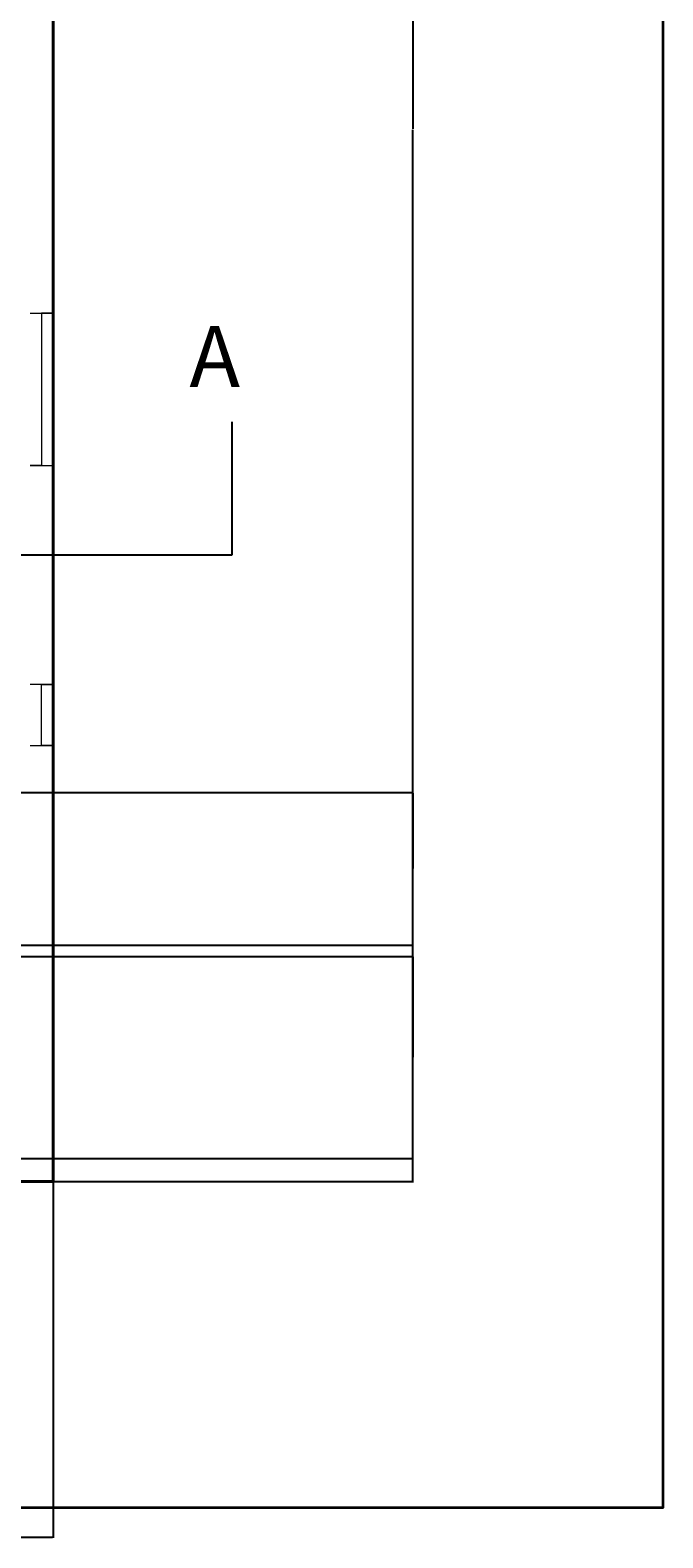
# Model space of a CAD drawing. Units: inches. Extents: x 1355 to 2746, y 1171 to 2751.
# Tile 15 of 24: x 2497 to 2746, y 1171 to 1764. Entities that reach past the tile are written whole.
import ezdxf

# ---------------------------------------------------------------- set-up
doc = ezdxf.new("R2010")
doc.units = ezdxf.units.IN
for name, color, linetype, lineweight in [('A-ANNO-DIMS', 2, 'Continuous', 18), ('A-ANNO-SYMB', 2, 'Continuous', 25), ('A-ANNO-TTLB', 7, 'Continuous', 35), ('A-GLAZ', 4, 'Continuous', 18), ('A-WALL', 7, 'Continuous', 40), ('A-WALL-PATT', 252, 'Continuous', 13)]:
    doc.layers.add(name, color=color, linetype=linetype, lineweight=lineweight)
doc.styles.get("Standard").update_dxf_attribs({"font": 'arial.ttf'})
doc.dimstyles.get("Standard").update_dxf_attribs({"dimtxt": 0.18, "dimasz": 0.18, "dimexe": 0.18, "dimexo": 0.0625, "dimgap": 0.09, "dimtad": 0, "dimtih": 1, "dimtoh": 1, "dimdec": 4, "dimzin": 0, "dimdsep": 46, "dimtxsty": 'Standard', "dimcen": 0.09, "dimadec": 0, "dimazin": 0, "dimtfac": 1, "dimtdec": 4, "dimtofl": 0, "dimtmove": 0, "dimatfit": 3, "dimfxl": 1, "dimtolj": 1, "dimtzin": 0, "dimarcsym": 0})

# ---------------------------------------------------------------- blocks, each defined once
blk = doc.blocks.new('WINDOW-PLAN-60')
for p, q in [((0, 60), (9, 60)), ((9, 60), (4.5, 60)), ((4.5, 60), (4.5, 0)), ((4.5, 0), (0, 0)), ((0, 0), (9, 0))]:
    blk.add_line(p, q)
blk = doc.blocks.new('WINDOW-PLAN-24-3')
for p, q in [((9, 24), (0, 24)), ((0, 24), (0, 24)), ((4.5, 0), (4.5, 24)), ((4.5, 24), (9, 24)), ((0, 0), (9, 0)), ((9, 0), (4.5, 0))]:
    blk.add_line(p, q)
blk = doc.blocks.new('*D97')
at = {"layer": 'A-ANNO-DIMS', "color": 0, "lineweight": -2, "transparency": 16777216}
for p, q in [((2080.39, 1311.24), (2080.39, 1171.06)), ((2506.39, 1311.24), (2506.39, 1171.06)), ((2080.57, 1171.24), (2293.1, 1171.24)), ((2506.21, 1171.24), (2293.68, 1171.24))]:
    blk.add_line(p, q, dxfattribs=at)
at = {"layer": 'A-ANNO-DIMS', "color": 0, "transparency": 16777216}
for points in [[(2080.57, 1171.27), (2080.57, 1171.21), (2080.39, 1171.24)], [(2506.21, 1171.27), (2506.21, 1171.21), (2506.39, 1171.24)]]:
    blk.add_solid(points, dxfattribs=at)
at = {"layer": 'Defpoints', "color": 0, "transparency": 16777216}
for p in [(2080.39, 1311.3), (2506.39, 1311.3), (2506.39, 1171.24)]:
    blk.add_point(p, dxfattribs=at)
at = {"layer": 'A-ANNO-DIMS', "color": 0, "transparency": 16777216, "insert": (2293.39, 1171.24), "char_height": 0.18, "attachment_point": 5}
blk.add_mtext('\\A1;426', dxfattribs=at)
blk = doc.blocks.new('*D98')
at = {"layer": 'A-ANNO-DIMS', "color": 0, "lineweight": -2, "transparency": 16777216}
for p, q in [((2506.45, 2139.3), (2648.07, 2139.3)), ((2647.89, 2139.12), (2647.89, 1725.48)), ((2647.89, 1311.48), (2647.89, 1725.12)), ((2506.45, 1311.3), (2648.07, 1311.3))]:
    blk.add_line(p, q, dxfattribs=at)
at = {"layer": 'A-ANNO-DIMS', "color": 0, "transparency": 16777216}
for points in [[(2647.86, 2139.12), (2647.92, 2139.12), (2647.89, 2139.3)], [(2647.86, 1311.48), (2647.92, 1311.48), (2647.89, 1311.3)]]:
    blk.add_solid(points, dxfattribs=at)
at = {"layer": 'Defpoints', "color": 0, "transparency": 16777216}
for p in [(2506.39, 2139.3), (2647.89, 2139.3), (2506.39, 1311.3)]:
    blk.add_point(p, dxfattribs=at)
at = {"layer": 'A-ANNO-DIMS', "color": 0, "transparency": 16777216, "insert": (2647.89, 1725.3), "char_height": 0.18, "attachment_point": 5}
blk.add_mtext('\\A1;828', dxfattribs=at)
blk = doc.blocks.new('*D126')
at = {"layer": 'A-ANNO-DIMS', "color": 0, "lineweight": -2, "transparency": 16777216}
for p, q in [((2080.39, 2219.34), (2080.39, 1171.06)), ((2506.39, 2219.34), (2506.39, 1171.06)), ((2080.57, 1171.24), (2293.1, 1171.24)), ((2506.21, 1171.24), (2293.68, 1171.24))]:
    blk.add_line(p, q, dxfattribs=at)
at = {"layer": 'A-ANNO-DIMS', "color": 0, "transparency": 16777216}
for points in [[(2080.57, 1171.27), (2080.57, 1171.21), (2080.39, 1171.24)], [(2506.21, 1171.27), (2506.21, 1171.21), (2506.39, 1171.24)]]:
    blk.add_solid(points, dxfattribs=at)
at = {"layer": 'Defpoints', "color": 0, "transparency": 16777216}
for p in [(2080.39, 2219.4), (2506.39, 2219.4), (2506.39, 1171.24)]:
    blk.add_point(p, dxfattribs=at)
at = {"layer": 'A-ANNO-DIMS', "color": 0, "transparency": 16777216, "insert": (2293.39, 1171.24), "char_height": 0.18, "attachment_point": 5}
blk.add_mtext('\\A1;426', dxfattribs=at)
blk = doc.blocks.new('*D142')
at = {"layer": 'A-ANNO-DIMS', "color": 0, "lineweight": -2, "transparency": 16777216}
for p, q in [((1931.77, 1399.8), (2648.07, 1399.8)), ((2647.89, 1399.62), (2647.89, 1360.23)), ((2647.89, 1320.48), (2647.89, 1359.87)), ((1931.77, 1320.3), (2648.07, 1320.3))]:
    blk.add_line(p, q, dxfattribs=at)
at = {"layer": 'A-ANNO-DIMS', "color": 0, "transparency": 16777216}
for points in [[(2647.86, 1399.62), (2647.92, 1399.62), (2647.89, 1399.8)], [(2647.86, 1320.48), (2647.92, 1320.48), (2647.89, 1320.3)]]:
    blk.add_solid(points, dxfattribs=at)
at = {"layer": 'Defpoints', "color": 0, "transparency": 16777216}
for p in [(1931.71, 1399.8), (2647.89, 1399.8), (1931.71, 1320.3)]:
    blk.add_point(p, dxfattribs=at)
at = {"layer": 'A-ANNO-DIMS', "color": 0, "transparency": 16777216, "insert": (2647.89, 1360.05), "char_height": 0.18, "attachment_point": 5}
blk.add_mtext('\\A1;79.5', dxfattribs=at)
blk = doc.blocks.new('*D143')
at = {"layer": 'A-ANNO-DIMS', "color": 0, "lineweight": -2, "transparency": 16777216}
for p, q in [((1931.77, 1464.3), (2648.07, 1464.3)), ((2647.89, 1464.12), (2647.89, 1434.48)), ((2647.89, 1404.48), (2647.89, 1434.12)), ((1931.77, 1404.3), (2648.07, 1404.3))]:
    blk.add_line(p, q, dxfattribs=at)
at = {"layer": 'A-ANNO-DIMS', "color": 0, "transparency": 16777216}
for points in [[(2647.86, 1464.12), (2647.92, 1464.12), (2647.89, 1464.3)], [(2647.86, 1404.48), (2647.92, 1404.48), (2647.89, 1404.3)]]:
    blk.add_solid(points, dxfattribs=at)
at = {"layer": 'Defpoints', "color": 0, "transparency": 16777216}
for p in [(1931.71, 1464.3), (2647.89, 1464.3), (1931.71, 1404.3)]:
    blk.add_point(p, dxfattribs=at)
at = {"layer": 'A-ANNO-DIMS', "color": 0, "transparency": 16777216, "insert": (2647.89, 1434.3), "char_height": 0.18, "attachment_point": 5}
blk.add_mtext('\\A1;60', dxfattribs=at)

msp = doc.modelspace()

# ---------------------------------------------------------------- hatches: boundary and pattern name
at = {"layer": 'A-WALL-PATT'}
h = msp.add_hatch(dxfattribs=at)
h.set_pattern_fill('ANSI32', color=256)
h.paths.add_polyline_path([(1660.2083, 2139.3018), (1614.5977, 2139.3018), (1614.5977, 2130.3018), (1655.7083, 2130.3018), (1655.7083, 1981.8018), (1660.2083, 1981.8018), (1660.2083, 2090.7225), (1692.5832, 2090.7225), (1692.5832, 2095.2225), (1660.2083, 2095.2225)])
h.paths.add_polyline_path([(1523.7083, 2130.3018), (1554.5977, 2130.3018), (1554.5977, 2134.8018), (1554.5977, 2139.3018), (1514.7083, 2139.3018), (1514.7083, 2071.8385), (1523.7083, 2071.8385)])
h.paths.add_polyline_path([(1940.7083, 2139.3018), (1883.7928, 2139.3018), (1883.7928, 2130.3018), (1931.7083, 2130.3018), (1931.7083, 2098.3333), (1940.7083, 2098.3333)])
h.paths.add_polyline_path([(1799.7083, 2130.3018), (1823.7928, 2130.3018), (1823.7928, 2134.8018), (1823.7928, 2139.3018), (1795.2083, 2139.3018), (1795.2083, 2130.3018), (1795.2083, 2095.2225), (1759.2134, 2095.2225), (1759.2134, 2090.7225), (1795.2083, 2090.7225), (1795.2083, 1981.8018), (1799.7083, 1981.8018), (1799.7083, 1986.3018)])
h.paths.add_polyline_path([(1940.7083, 2038.3333), (1931.7083, 2038.3333), (1931.7083, 1986.3018), (1832.7083, 1986.3018), (1832.7083, 1947.1338), (1837.2083, 1947.1338), (1837.2083, 1981.8018), (1931.7083, 1981.8018), (1931.7083, 1967.1939), (1940.7083, 1967.1939)])
h.paths.add_polyline_path([(1940.7083, 1943.1939), (1931.7083, 1943.1939), (1931.7083, 1921.8018), (1837.2083, 1921.8018), (1837.2083, 1926.0511), (1832.7083, 1926.0511), (1832.7083, 1917.3018), (1931.7083, 1917.3018), (1931.7083, 1908.3321), (1940.7083, 1908.3321)])
h.paths.add_polyline_path([(1940.7083, 1884.3321), (1931.7083, 1884.3321), (1931.7083, 1869.3018), (1899.4583, 1869.3018), (1899.4583, 1864.8018), (1931.7083, 1864.8018), (1931.7083, 1773.3018), (1786.5143, 1773.3018), (1786.5143, 1764.3018), (1844.7083, 1764.3018), (1844.7083, 1748.9343), (1853.7083, 1748.9343), (1853.7083, 1764.3018), (1931.7083, 1764.3018), (1931.7083, 1652.9424), (1940.7083, 1652.9424)])
h.paths.add_polyline_path([(1799.7083, 1864.8018), (1806.0522, 1864.8018), (1806.0522, 1867.0518), (1806.0522, 1869.3018), (1799.7083, 1869.3018), (1799.7083, 1917.3018), (1799.7083, 1921.8018), (1795.2083, 1921.8018), (1795.2083, 1773.3018), (1799.7083, 1773.3018)])
h.paths.add_polyline_path([(1872.8988, 1867.0518), (1872.8988, 1869.3018), (1867.2083, 1869.3018), (1867.2083, 1917.3018), (1862.7083, 1917.3018), (1862.7083, 1869.3018), (1836.9546, 1869.3018), (1836.9546, 1864.8018), (1862.7083, 1864.8018), (1872.8988, 1864.8018)])
h.paths.add_polyline_path([(1749.2197, 1773.3018), (1655.7083, 1773.3018), (1523.7083, 1773.3018), (1523.7083, 1828.4963), (1514.7083, 1828.4963), (1514.7083, 1753.9033), (1519.2083, 1753.9033), (1523.7083, 1753.9033), (1523.7083, 1764.3018), (1655.7083, 1764.3018), (1749.2197, 1764.3018), (1749.2197, 1768.8018)])
h.paths.add_polyline_path([(1660.2083, 1921.8018), (1655.7083, 1921.8018), (1655.7083, 1917.3018), (1655.7083, 1773.3018), (1660.2083, 1773.3018)])
h.paths.add_polyline_path([(1523.7083, 2011.8385), (1514.7083, 2011.8385), (1514.7083, 1973.114), (1519.2083, 1973.114), (1523.7083, 1973.114), (1523.7083, 1976.8227), (1523.7083, 1981.8018), (1618.2083, 1981.8018), (1618.2083, 1921.8018), (1553.707, 1921.8018), (1553.707, 1917.3018), (1622.7083, 1917.3018), (1622.7083, 1919.5518), (1622.7083, 1921.8018), (1622.7083, 1986.3018), (1523.7083, 1986.3018)])
h.paths.add_polyline_path([(1529.6686, 1919.5518), (1529.6686, 1921.8018), (1523.7083, 1921.8018), (1523.7083, 1949.114), (1514.7083, 1949.114), (1514.7083, 1888.4963), (1523.7083, 1888.4963), (1523.7083, 1917.3018), (1529.6686, 1917.3018)])
h.paths.add_polyline_path([(1538.9419, 1775.643), (1585.5504, 1775.643), (1585.5504, 1798.0318), (1538.9419, 1798.0318)], flags=25)
h.paths.add_polyline_path([(1696.7097, 1497.3356), (1769.5651, 1497.3356), (1769.5651, 1523.4559), (1696.7097, 1523.4559)], flags=9)
h.paths.add_polyline_path([(1629.1643, 1230.5133), (1877.0879, 1230.5133), (1877.0879, 1267.606), (1629.1643, 1267.606)], flags=9)
h.paths.add_polyline_path([(2533.4462, 2215.4033), (2579.9292, 2215.4033), (2579.9292, 2231.889), (2533.4462, 2231.889)], flags=9)
h.paths.add_polyline_path([(2540.822, 2515.6945), (2594.2245, 2515.6945), (2594.2245, 2545.5463), (2540.822, 2545.5463)], flags=9)
h.paths.add_polyline_path([(2535.9857, 2588.2819), (2582.4687, 2588.2819), (2582.4687, 2604.7675), (2535.9857, 2604.7675)], flags=9)
h.paths.add_polyline_path([(2537.1627, 2617.1172), (2649.1245, 2617.1172), (2649.1245, 2633.6029), (2537.1627, 2633.6029)], flags=9)
h.paths.add_polyline_path([(2218.0051, 2168.228), (2363.9573, 2168.228), (2363.9573, 2205.3208), (2218.0051, 2205.3208)], flags=9)
h.paths.add_polyline_path([(1650.2156, 2165.3631), (1800.3547, 2165.3631), (1800.3547, 2202.4559), (1650.2156, 2202.4559)], flags=9)
h.paths.add_polyline_path([(2553.9592, 1610.7663), (2588.4203, 1610.7663), (2588.4203, 1660.2233), (2553.9592, 1660.2233)], flags=9)
h.paths.add_polyline_path([(1549.0868, 1648.2033), (1595.6952, 1648.2033), (1595.6952, 1670.5921), (1549.0868, 1670.5921)], flags=9)
h.paths.add_polyline_path([(1546.9525, 1502.0931), (1583.3413, 1502.0931), (1583.3413, 1524.4819), (1546.9525, 1524.4819)], flags=9)
h.paths.add_polyline_path([(1540.7704, 1433.4431), (1587.3788, 1433.4431), (1587.3788, 1455.8319), (1540.7704, 1455.8319)], flags=9)
h.paths.add_polyline_path([(1683.6524, 1321.5269), (1760.6169, 1321.5269), (1760.6169, 1333.8911), (1683.6524, 1333.8911)], flags=9)
h.paths.add_polyline_path([(1832.0485, 1356.0874), (1873.0989, 1356.0874), (1873.0989, 1378.4762), (1832.0485, 1378.4762)], flags=9)
h.paths.add_polyline_path([(1877.9694, 1431.2138), (1926.3827, 1431.2138), (1926.3827, 1453.578), (1877.9694, 1453.578)], flags=9)
h.paths.add_polyline_path([(1847.3106, 1499.8371), (1883.6994, 1499.8371), (1883.6994, 1522.2259), (1847.3106, 1522.2259)], flags=9)
h.paths.add_polyline_path([(1813.7015, 1640.7287), (1860.3099, 1640.7287), (1860.3099, 1663.1175), (1813.7015, 1663.1175)], flags=9)
h.paths.add_polyline_path([(1876.2576, 1710.2471), (1912.9452, 1710.2471), (1912.9452, 1732.6359), (1876.2576, 1732.6359)], flags=25)
h.paths.add_polyline_path([(1695.9163, 1715.3064), (1736.9668, 1715.3064), (1736.9668, 1737.6952), (1695.9163, 1737.6952)], flags=9)
h.paths.add_polyline_path([(1881.8583, 1888.9094), (1930.2717, 1888.9094), (1930.2717, 1911.2737), (1881.8583, 1911.2737)], flags=9)
h.paths.add_polyline_path([(1823.9298, 1798.6431), (1864.9803, 1798.6431), (1864.9803, 1821.0319), (1823.9298, 1821.0319)], flags=25)
h.paths.add_polyline_path([(1845.6062, 1948.1408), (1881.995, 1948.1408), (1881.995, 1970.5296), (1845.6062, 1970.5296)], flags=25)
h.paths.add_polyline_path([(1849.027, 1991.5151), (1895.6355, 1991.5151), (1895.6355, 2013.9039), (1849.027, 2013.9039)], flags=25)
h.paths.add_polyline_path([(1684.9725, 2113.8416), (1764.2658, 2113.8416), (1764.2658, 2126.2058), (1684.9725, 2126.2058)], flags=9)
h.paths.add_polyline_path([(1688.6193, 1913.0676), (1776.2005, 1913.0676), (1776.2005, 1935.4564), (1688.6193, 1935.4564)], flags=9)
h.paths.add_polyline_path([(1571.4689, 1930.9816), (1607.8577, 1930.9816), (1607.8577, 1953.3704), (1571.4689, 1953.3704)], flags=25)
h.paths.add_polyline_path([(1535.3581, 1998.3125), (1581.9665, 1998.3125), (1581.9665, 2020.7014), (1535.3581, 2020.7014)], flags=9)
h = msp.add_hatch(dxfattribs=at)
h.set_pattern_fill('ANSI32', color=256)
h.paths.add_polyline_path([(1749.2197, 1686.3018), (1732.6892, 1686.3018), (1523.7083, 1686.3018), (1523.7083, 1705.9033), (1514.7083, 1705.9033), (1514.7083, 1647.8732), (1519.2083, 1647.8732), (1523.7083, 1647.8732), (1523.7083, 1677.3018), (1655.7083, 1677.3018), (1655.7083, 1528.8018), (1660.2083, 1528.8018), (1660.2083, 1677.3018), (1732.6892, 1677.3018), (1749.2197, 1677.3018)])
h.paths.add_polyline_path([(1931.7083, 1686.3018), (1853.7083, 1686.3018), (1853.7083, 1703.5696), (1844.7083, 1703.5696), (1844.7083, 1686.3018), (1788.0274, 1686.3018), (1788.0274, 1677.3018), (1795.2083, 1677.3018), (1795.2083, 1528.8018), (1799.7083, 1528.8018), (1799.7083, 1677.3018), (1844.7083, 1677.3018), (1931.7083, 1677.3018)])
h.paths.add_polyline_path([(1931.7083, 1533.3018), (1844.7083, 1533.3018), (1832.7083, 1533.3018), (1832.7083, 1531.0518), (1832.7083, 1528.8018), (1832.7083, 1495.7519), (1837.2083, 1495.7519), (1837.2083, 1528.8018), (1931.7083, 1528.8018)])
h.paths.add_polyline_path([(1940.7083, 1592.9424), (1931.7083, 1592.9424), (1931.7083, 1506.7845), (1940.7083, 1506.7845)])
h.paths.add_polyline_path([(1940.7083, 1482.7845), (1936.2083, 1482.7845), (1931.7083, 1482.7845), (1931.7083, 1320.3018), (1880.7083, 1320.3018), (1880.7083, 1311.3018), (1940.7083, 1311.3018)])
h.paths.add_polyline_path([(1931.7083, 1468.8018), (1844.7083, 1468.8018), (1837.2083, 1468.8018), (1837.2083, 1474.34), (1832.7083, 1474.34), (1832.7083, 1468.8018), (1832.7083, 1464.3018), (1844.7083, 1464.3018), (1931.7083, 1464.3018)])
h.paths.add_polyline_path([(1863.8571, 1464.3018), (1859.3571, 1464.3018), (1859.3571, 1404.1662), (1838.1542, 1404.1662), (1838.1542, 1399.8018), (1869.4185, 1399.8018), (1869.4185, 1402.0518), (1869.4185, 1404.3018), (1863.8571, 1404.3018)])
h.paths.add_polyline_path([(1799.7083, 1399.6662), (1805.4082, 1399.6662), (1805.4082, 1401.9162), (1805.4082, 1404.1662), (1799.7083, 1404.1662), (1799.7083, 1464.3018), (1799.7083, 1468.8018), (1795.2083, 1468.8018), (1795.2083, 1356.2098), (1761.2597, 1356.2098), (1761.2597, 1351.7098), (1795.2083, 1351.7098), (1795.2083, 1320.3018), (1795.2083, 1311.3018), (1844.7083, 1311.3018), (1844.7083, 1315.8018), (1844.7083, 1320.3018), (1799.7083, 1320.3018)])
h.paths.add_polyline_path([(1692.9218, 1356.2098), (1660.2083, 1356.2098), (1660.2083, 1430.786), (1657.9583, 1430.786), (1655.7083, 1430.786), (1655.7083, 1320.3018), (1611.934, 1320.3018), (1611.934, 1311.3018), (1660.2083, 1311.3018), (1660.2083, 1351.7098), (1692.9218, 1351.7098)])
h.paths.add_polyline_path([(1523.7083, 1372.653), (1514.7083, 1372.653), (1514.7083, 1311.3018), (1551.934, 1311.3018), (1551.934, 1315.8018), (1551.934, 1320.3018), (1523.7083, 1320.3018)])
h.paths.add_polyline_path([(1523.7083, 1490.9023), (1514.7083, 1490.9023), (1514.7083, 1432.653), (1519.2083, 1432.653), (1523.7083, 1432.653)])
h.paths.add_polyline_path([(1660.2083, 1468.8018), (1622.7083, 1468.8018), (1622.7083, 1473.1566), (1618.2083, 1473.1566), (1618.2083, 1468.8018), (1523.7083, 1468.8018), (1523.7083, 1464.3018), (1655.7083, 1464.3018), (1655.7083, 1460.5634), (1660.2083, 1460.5634)])
h.paths.add_polyline_path([(1523.7083, 1587.8732), (1514.7083, 1587.8732), (1514.7083, 1514.9023), (1519.2083, 1514.9023), (1523.7083, 1514.9023)])
h.paths.add_polyline_path([(1622.7083, 1533.3018), (1523.7083, 1533.3018), (1523.7083, 1528.8018), (1618.2083, 1528.8018), (1618.2083, 1494.4205), (1622.7083, 1494.4205), (1622.7083, 1528.8018)])
h.paths.add_polyline_path([(1696.7097, 1497.3356), (1769.5651, 1497.3356), (1769.5651, 1523.4559), (1696.7097, 1523.4559)], flags=9)
h.paths.add_polyline_path([(1629.1643, 1230.5133), (1877.0879, 1230.5133), (1877.0879, 1267.606), (1629.1643, 1267.606)], flags=9)
h.paths.add_polyline_path([(2533.4462, 2215.4033), (2579.9292, 2215.4033), (2579.9292, 2231.889), (2533.4462, 2231.889)], flags=9)
h.paths.add_polyline_path([(2540.822, 2515.6945), (2594.2245, 2515.6945), (2594.2245, 2545.5463), (2540.822, 2545.5463)], flags=9)
h.paths.add_polyline_path([(2535.9857, 2588.2819), (2582.4687, 2588.2819), (2582.4687, 2604.7675), (2535.9857, 2604.7675)], flags=9)
h.paths.add_polyline_path([(2537.1627, 2617.1172), (2649.1245, 2617.1172), (2649.1245, 2633.6029), (2537.1627, 2633.6029)], flags=9)
h.paths.add_polyline_path([(2218.0051, 2168.228), (2363.9573, 2168.228), (2363.9573, 2205.3208), (2218.0051, 2205.3208)], flags=9)
h.paths.add_polyline_path([(1650.2156, 2165.3631), (1800.3547, 2165.3631), (1800.3547, 2202.4559), (1650.2156, 2202.4559)], flags=9)
h.paths.add_polyline_path([(2553.9592, 1610.7663), (2588.4203, 1610.7663), (2588.4203, 1660.2233), (2553.9592, 1660.2233)], flags=9)
h.paths.add_polyline_path([(1549.0868, 1648.2033), (1595.6952, 1648.2033), (1595.6952, 1670.5921), (1549.0868, 1670.5921)], flags=25)
h.paths.add_polyline_path([(1546.9525, 1502.0931), (1583.3413, 1502.0931), (1583.3413, 1524.4819), (1546.9525, 1524.4819)], flags=25)
h.paths.add_polyline_path([(1540.7704, 1433.4431), (1587.3788, 1433.4431), (1587.3788, 1455.8319), (1540.7704, 1455.8319)], flags=9)
h.paths.add_polyline_path([(1683.6524, 1321.5269), (1760.6169, 1321.5269), (1760.6169, 1333.8911), (1683.6524, 1333.8911)], flags=9)
h.paths.add_polyline_path([(1832.0485, 1356.0874), (1873.0989, 1356.0874), (1873.0989, 1378.4762), (1832.0485, 1378.4762)], flags=9)
h.paths.add_polyline_path([(1877.9694, 1431.2138), (1926.3827, 1431.2138), (1926.3827, 1453.578), (1877.9694, 1453.578)], flags=9)
h.paths.add_polyline_path([(1847.3106, 1499.8371), (1883.6994, 1499.8371), (1883.6994, 1522.2259), (1847.3106, 1522.2259)], flags=25)
h.paths.add_polyline_path([(1813.7015, 1640.7287), (1860.3099, 1640.7287), (1860.3099, 1663.1175), (1813.7015, 1663.1175)], flags=25)
h.paths.add_polyline_path([(1876.2576, 1710.2471), (1912.9452, 1710.2471), (1912.9452, 1732.6359), (1876.2576, 1732.6359)], flags=9)
h.paths.add_polyline_path([(1695.9163, 1715.3064), (1736.9668, 1715.3064), (1736.9668, 1737.6952), (1695.9163, 1737.6952)], flags=9)
h.paths.add_polyline_path([(1881.8583, 1888.9094), (1930.2717, 1888.9094), (1930.2717, 1911.2737), (1881.8583, 1911.2737)], flags=9)
h.paths.add_polyline_path([(1823.9298, 1798.6431), (1864.9803, 1798.6431), (1864.9803, 1821.0319), (1823.9298, 1821.0319)], flags=9)
h.paths.add_polyline_path([(1845.6062, 1948.1408), (1881.995, 1948.1408), (1881.995, 1970.5296), (1845.6062, 1970.5296)], flags=9)
h.paths.add_polyline_path([(1849.027, 1991.5151), (1895.6355, 1991.5151), (1895.6355, 2013.9039), (1849.027, 2013.9039)], flags=9)
h.paths.add_polyline_path([(1684.9725, 2113.8416), (1764.2658, 2113.8416), (1764.2658, 2126.2058), (1684.9725, 2126.2058)], flags=9)
h.paths.add_polyline_path([(1688.6193, 1913.0676), (1776.2005, 1913.0676), (1776.2005, 1935.4564), (1688.6193, 1935.4564)], flags=9)
h.paths.add_polyline_path([(1538.9419, 1775.643), (1585.5504, 1775.643), (1585.5504, 1798.0318), (1538.9419, 1798.0318)], flags=9)
h.paths.add_polyline_path([(1571.4689, 1930.9816), (1607.8577, 1930.9816), (1607.8577, 1953.3704), (1571.4689, 1953.3704)], flags=9)
h.paths.add_polyline_path([(1535.3581, 1998.3125), (1581.9665, 1998.3125), (1581.9665, 2020.7014), (1535.3581, 2020.7014)], flags=9)

# ---------------------------------------------------------------- linework, layer by layer
at = {"layer": 'A-ANNO-SYMB'}
for p, q in [((2576.886, 1557.845), (2576.886, 1610.2283)), ((2031.1535, 1557.845), (2576.886, 1557.845))]:
    msp.add_line(p, q, dxfattribs=at)
at = {"layer": 'A-ANNO-TTLB'}
msp.add_lwpolyline([(1355.0901, 2751.4741), (2746.1804, 2751.4741), (2746.1804, 1182.883), (1355.0901, 1182.883)], close=True, dxfattribs=at)
at = {"layer": 'A-WALL'}
for p, q in [((2506.3909, 2139.3018), (2506.3909, 1311.3018)), ((2506.3909, 1311.3018), (2360.8909, 1311.3018))]:
    msp.add_line(p, q, dxfattribs=at)

# ---------------------------------------------------------------- block references
at = {"layer": 'A-GLAZ'}
for name, p in [('WINDOW-PLAN-60', (2497.3906, 1592.9421)), ('WINDOW-PLAN-24-3', (2497.3906, 1482.784))]:
    msp.add_blockref(name, p, dxfattribs=at)

# ---------------------------------------------------------------- texts
at = {"layer": 'A-ANNO-SYMB', "insert": (2560.0083, 1647.8713), "char_height": 24, "attachment_point": 1}
msp.add_mtext_dynamic_manual_height_columns('A', width=14.965607, gutter_width=12.5, heights=[0], dxfattribs=at)

# ---------------------------------------------------------------- dimensions: what is measured, and where the dimension line sits
at = {"layer": 'A-ANNO-DIMS'}
for p1, p2, picture in [((2080.3909, 2219.3999), (2506.3909, 2219.3999), '*D126'), ((2080.3909, 1311.3018), (2506.3909, 1311.3018), '*D97')]:
    dim = msp.add_linear_dim(base=(2506.3909, 1171.2388), p1=p1, p2=p2, dimstyle='Standard', override={"dimdec": 0, "dimlfac": 1, "dimrnd": 0, "dimzin": 0, "dimdsep": 46, "dimlunit": 2}, dxfattribs=at)
    dim.commit()
    dim.dimension.update_dxf_attribs({"geometry": picture, "text_midpoint": (2293.3909, 1171.2388)})
for base, p1, p2, override, picture, middle in [((2647.886, 2139.3018), (2506.3909, 1311.3018), (2506.3909, 2139.3018), {"dimdec": 0, "dimlfac": 1, "dimrnd": 0, "dimzin": 0, "dimdsep": 46, "dimlunit": 2}, '*D98', (2647.886, 1725.3018)), ((2647.886, 1464.3018), (1931.7083, 1404.3018), (1931.7083, 1464.3018), {"dimdec": 0, "dimlfac": 1, "dimrnd": 0, "dimzin": 0, "dimdsep": 46, "dimlunit": 2}, '*D143', (2647.886, 1434.3018)), ((2647.886, 1399.8018), (1931.7083, 1320.3018), (1931.7083, 1399.8018), {"dimdec": 1, "dimlfac": 1, "dimrnd": 0, "dimzin": 0, "dimdsep": 46, "dimlunit": 2}, '*D142', (2647.886, 1360.0518))]:
    dim = msp.add_linear_dim(base=base, p1=p1, p2=p2, angle=90, dimstyle='Standard', override=override, dxfattribs=at)
    dim.commit()
    dim.dimension.update_dxf_attribs({"geometry": picture, "text_midpoint": middle})

doc.saveas('drawing.dxf')
